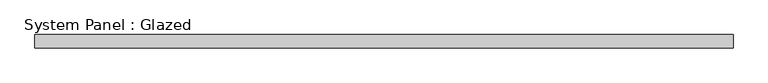
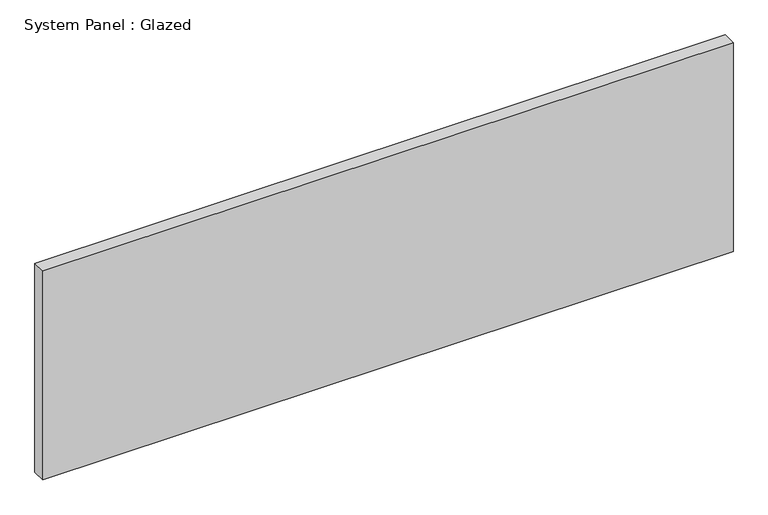
"""IFC4 building model written with IfcOpenShell, lengths in millimetres: plate geometry, System Panel : Glazed."""

from ifc_helpers import new_model, si_unit, origin, origin_with_axes, place, context, project, spatial, polyline, outline, extrude, source, transform, mapped, element, save


def system_panel_glazed_cff82037(model_context):
    return source(origin(), model_context, "Body", "SweptSolid", [
        extrude(outline(polyline([(654.0499999, 19.05), (-654.0499999, 19.05), (-654.0499999, 44.45), (654.0499999, 44.45), (654.0499999, 19.05)])), origin_with_axes(), (0.0, 0.0, 1.0), 419.1),
    ])


if __name__ == "__main__":
    model = new_model("IFC4")
    model_context = context("Model", 3, world=origin())
    ifc_project = project(units=[si_unit("LENGTHUNIT", "METRE", prefix="MILLI")], contexts=[model_context])
    site = spatial("IfcSite", under=ifc_project)
    building = spatial("IfcBuilding", under=site)
    placement = place(None, origin())
    system_panel_glazed_shape = system_panel_glazed_cff82037(model_context)
    element("IfcPlate", 1, ObjectType="System Panel : Glazed", at=placement, inside=building, context=model_context, shape_type="MappedRepresentation", body=[
        mapped(system_panel_glazed_shape, transform((0.0, 0.0, 0.0), x_axis=(1.0, 0.0, 0.0), y_axis=(0.0, 1.0, 0.0), z_axis=(0.0, 0.0, 1.0))),
    ])
    save(model, "model.ifc")

# Revit data of these elements
# Type "System Panel : Glazed"
#   Construction Type Id = "GSP4R"
#   Analytic Construction = "1/8 in Pilkington single glazing"
#   Visual Light Transmittance = 0.9
#   Solar Heat Gain Coefficient = 0.86
#   Heat Transfer Coefficient (U) = 1.18115 BTU/(h·ft²·°F)
#   Define Thermal Properties by = 1
# Element 1 (IfcPlate, "System Panel : Glazed")
#   Materials on its faces: "glass panel 223"
# Materials
#   "glass panel 223": class "Generic", colour RGB 120 120 120, transparency 0, Cost = 0
